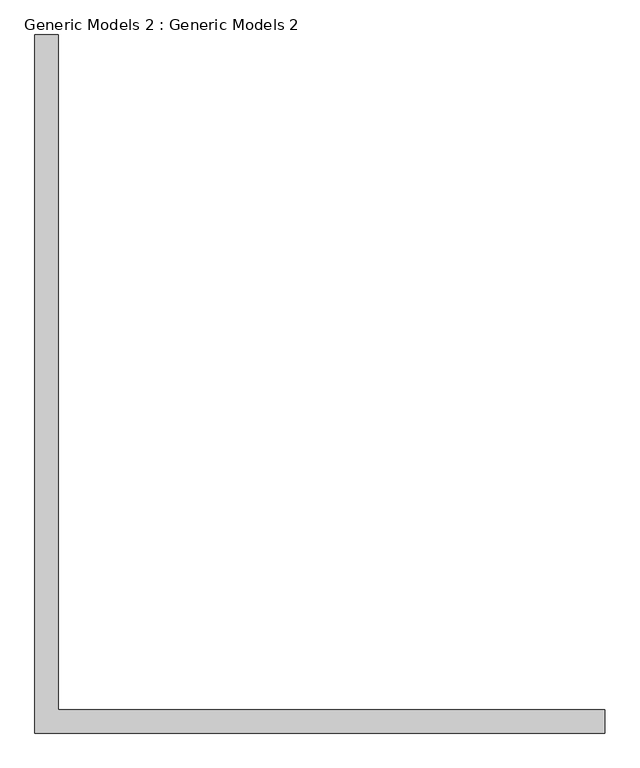
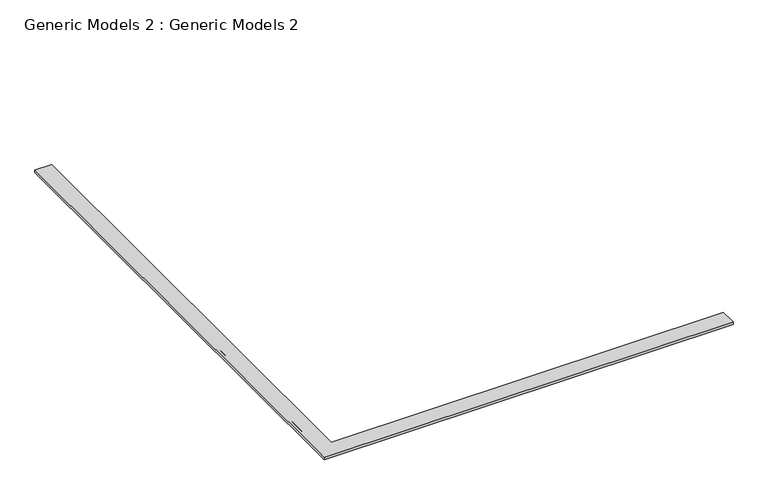
"""IFC4 building model written with IfcOpenShell, lengths in millimetres: proxy geometry, Generic Models 2 : Generic Models 2."""

from ifc_helpers import new_model, si_unit, frame, origin, place, context, project, spatial, circle_curve, ellipse_curve, source, transform, mapped, element, save
from ifc_brep_helpers import plane_surface, cylinder_surface, advanced_brep


def generic_models_2_generic_models_2_85994228(model_context):
    return source(origin(), model_context, "Body", "AdvancedBrep", [
        advanced_brep(
        [(-7911.9236584, -13805.302305, 3352.8), (-7911.9236584, -13805.302305, 3327.4), (-7911.9236584, -13773.552305, 3327.4), (-7911.9236584, -13773.552305, 3308.35), (-7911.9236584, -13754.502305, 3308.35), (-7911.9236584, -13754.502305, 3295.65), (-7911.9236584, -13735.452305, 3295.65), (-7911.9236584, -13671.952305, 3263.9), (-7911.9236584, -13671.952305, 3251.2), (-7911.9236584, -13640.202305, 3251.2), (-7911.9236584, -13640.202305, 3352.8), (-11796.2293601, -13640.202305, 3251.2), (-11796.2293601, -13640.202305, 3352.8), (-11796.2293601, -8842.6396616, 3352.8), (-11961.3293601, -8842.6396616, 3352.8), (-11961.3293601, -13805.302305, 3352.8), (-11796.2293601, -8842.6396616, 3251.2), (-11827.9793601, -8842.6396616, 3251.2), (-11827.9793601, -8842.6396616, 3263.9), (-11891.4793601, -8842.6396616, 3295.65), (-11910.5293601, -8842.6396616, 3295.65), (-11910.5293601, -8842.6396616, 3308.35), (-11929.5793601, -8842.6396616, 3308.35), (-11929.5793601, -8842.6396616, 3327.4), (-11961.3293601, -8842.6396616, 3327.4), (-11961.3293601, -13805.302305, 3327.4), (-11929.5793601, -13773.552305, 3327.4), (-11929.5793601, -13773.552305, 3308.35), (-11910.5293601, -13754.502305, 3308.35), (-11910.5293601, -13754.502305, 3295.65), (-11891.4793601, -13735.452305, 3295.65), (-11827.9793601, -13671.952305, 3263.9), (-11827.9793601, -13671.952305, 3251.2)],
        [
            (0, 1),
            (1, 2),
            (2, 3),
            (3, 4),
            (4, 5),
            (5, 6),
            (6, 7, circle_curve(frame((-7911.9236584, -13688.0269583, 3311.1256934), z_axis=(1.0, 0.0, 0.0), x_axis=(0.0, -1.0, 0.0)), 49.8864771)),
            (7, 8),
            (8, 9),
            (9, 10),
            (10, 0),
            (9, 11),
            (11, 12),
            (12, 10),
            (12, 13),
            (13, 14),
            (14, 15),
            (15, 0),
            (13, 16),
            (16, 17),
            (17, 18),
            (18, 19, circle_curve(frame((-11844.0540134, -8842.6396616, 3311.1256934), z_axis=(0.0, 1.0, 0.0), x_axis=(-1.0, 0.0, 0.0)), 49.8864771)),
            (19, 20),
            (20, 21),
            (21, 22),
            (22, 23),
            (23, 24),
            (24, 14),
            (11, 16),
            (15, 25),
            (25, 1),
            (25, 24),
            (23, 26),
            (26, 2),
            (26, 27),
            (27, 3),
            (27, 22),
            (21, 28),
            (28, 4),
            (28, 29),
            (29, 5),
            (29, 20),
            (19, 30),
            (30, 6),
            (30, 31, ellipse_curve(frame((-11844.0540134, -13688.0269583, 3311.1256934), z_axis=(0.7071067811865457, -0.7071067811865492, 0.0), x_axis=(0.7071067811865495, 0.7071067811865456, 0.0)), 70.5501324, 49.8864771)),
            (31, 7),
            (31, 32),
            (32, 8),
            (32, 17),
            (18, 31),
        ],
        [
            plane_surface(frame((-7911.9236584, -13640.202305, 3352.8), z_axis=(1.0, 0.0, 0.0), x_axis=(0.0, 0.0, 1.0))),
            plane_surface(frame((-7911.9236584, -13640.202305, 3251.2), z_axis=(0.0, 1.0, 0.0), x_axis=(-1.0, 0.0, 0.0))),
            plane_surface(frame((-7911.9236584, -13640.202305, 3352.8), z_axis=(0.0, 0.0, 1.0), x_axis=(-1.0, 0.0, 0.0))),
            plane_surface(frame((-11796.2293601, -8842.6396616, 3352.8), z_axis=(0.0, 1.0, 0.0), x_axis=(0.0, 0.0, 1.0))),
            plane_surface(frame((-11796.2293601, -13640.202305, 3251.2), z_axis=(1.0, 0.0, 0.0), x_axis=(0.0, 1.0, 0.0))),
            plane_surface(frame((-7911.9236584, -13805.302305, 3352.8), z_axis=(0.0, -1.0, 0.0), x_axis=(-1.0, 0.0, 0.0))),
            plane_surface(frame((-7911.9236584, -13805.302305, 3327.4), z_axis=(0.0, 0.0, -1.0), x_axis=(-1.0, 0.0, 0.0))),
            plane_surface(frame((-7911.9236584, -13773.552305, 3327.4), z_axis=(0.0, -1.0, -1.0169136580860064e-12), x_axis=(-1.0, 0.0, 0.0))),
            plane_surface(frame((-7911.9236584, -13773.552305, 3308.35), z_axis=(0.0, 1.0114600803129775e-12, -1.0), x_axis=(-1.0, 0.0, 0.0))),
            plane_surface(frame((-7911.9236584, -13754.502305, 3308.35), z_axis=(0.0, -1.0, -1.0494708216981705e-12), x_axis=(-1.0, 0.0, 0.0))),
            plane_surface(frame((-7911.9236584, -13754.502305, 3295.65), z_axis=(0.0, 1.0442051053225801e-12, -1.0), x_axis=(-1.0, 0.0, 0.0))),
            cylinder_surface(frame((-7911.9236584, -13688.0269583, 3311.1256934), z_axis=(1.0, 0.0, 0.0), x_axis=(0.0, -1.0, 0.0)), 49.8864771),
            plane_surface(frame((-7911.9236584, -13671.952305, 3263.9), z_axis=(0.0, -1.0, 0.0), x_axis=(-1.0, 0.0, 0.0))),
            plane_surface(frame((-7911.9236584, -13671.952305, 3251.2), z_axis=(0.0, 0.0, -1.0), x_axis=(-1.0, 0.0, 0.0))),
            plane_surface(frame((-11961.3293601, -13805.302305, 3352.8), z_axis=(-1.0, 0.0, 0.0), x_axis=(0.0, 1.0, 0.0))),
            plane_surface(frame((-11929.5793601, -13773.552305, 3327.4), z_axis=(-1.0, 0.0, -1.0169136580860064e-12), x_axis=(0.0, 1.0, 0.0))),
            plane_surface(frame((-11910.5293601, -13754.502305, 3308.35), z_axis=(-1.0, 0.0, -1.0494708216981705e-12), x_axis=(0.0, 1.0, 0.0))),
            cylinder_surface(frame((-11844.0540134, -13640.202305, 3311.1256934), z_axis=(0.0, -1.0, 0.0), x_axis=(-1.0, 0.0, 0.0)), 49.8864771),
            plane_surface(frame((-11827.9793601, -13671.952305, 3263.9), z_axis=(-1.0, 0.0, 0.0), x_axis=(0.0, 1.0, 0.0))),
        ],
        [
            (0, [[1, 2, 3, 4, 5, 6, 7, 8, 9, 10, 11]]),
            (1, [[-10, 12, 13, 14]]),
            (2, [[-11, -14, 15, 16, 17, 18]]),
            (3, [[-16, 19, 20, 21, 22, 23, 24, 25, 26, 27, 28]]),
            (4, [[-13, 29, -19, -15]]),
            (5, [[-1, -18, 30, 31]]),
            (6, [[-2, -31, 32, -27, 33, 34]]),
            (7, [[-3, -34, 35, 36]]),
            (8, [[-4, -36, 37, -25, 38, 39]]),
            (9, [[-5, -39, 40, 41]]),
            (10, [[-6, -41, 42, -23, 43, 44]]),
            (11, [[-7, -44, 45, 46]]),
            (12, [[-8, -46, 47, 48]]),
            (13, [[-9, -48, 49, -20, -29, -12]]),
            (14, [[-30, -17, -28, -32]]),
            (15, [[-35, -33, -26, -37]]),
            (16, [[-40, -38, -24, -42]]),
            (17, [[-45, -43, -22, 50]]),
            (18, [[-47, -50, -21, -49]]),
        ],
    ),
    ])


if __name__ == "__main__":
    model = new_model("IFC4")
    model_context = context("Model", 3, world=origin())
    ifc_project = project(units=[si_unit("LENGTHUNIT", "METRE", prefix="MILLI")], contexts=[model_context])
    site = spatial("IfcSite", under=ifc_project)
    building = spatial("IfcBuilding", under=site)
    placement = place(None, origin())
    generic_models_2_generic_models_2_shape = generic_models_2_generic_models_2_85994228(model_context)
    element("IfcBuildingElementProxy", 1, Name="Generic Models 2 : Generic Models 2", ObjectType="Generic Models 2 : Generic Models 2", at=placement, inside=building, context=model_context, shape_type="MappedRepresentation", body=[
        mapped(generic_models_2_generic_models_2_shape, transform((0.0, 0.0, 0.0), x_axis=(1.0, 0.0, 0.0), y_axis=(0.0, 1.0, 0.0), z_axis=(0.0, 0.0, 1.0))),
    ])
    save(model, "model.ifc")

# Revit data of these elements
# Element 1 (IfcBuildingElementProxy, "Generic Models 2 : Generic Models 2")
#   Materials on its faces: "white colour"
# Materials
#   "white colour": class "Generic", colour RGB 120 120 120, transparency 0, Cost = 0
